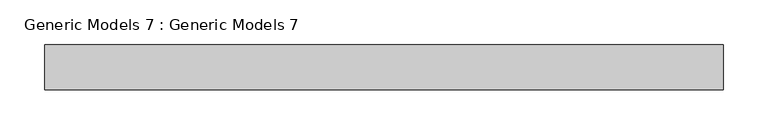
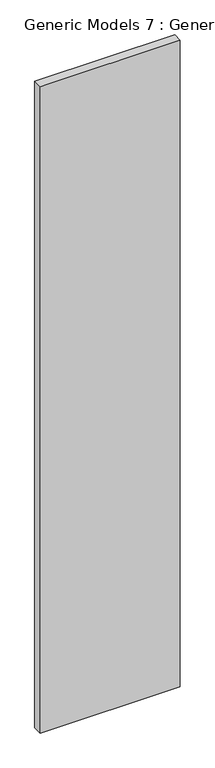
"""IFC4 building model written with IfcOpenShell, lengths in millimetres: proxy geometry, Generic Models 7 : Generic Models 7."""

from ifc_helpers import new_model, si_unit, frame, origin, place, context, project, spatial, polyline, outline, extrude, source, transform, mapped, element, save


def generic_models_7_generic_models_7_c575a30d(model_context):
    return source(origin(), model_context, "Body", "SweptSolid", [
        extrude(outline(polyline([(-5810.3607439, -6392.6842658), (-6572.3607439, -6392.6842658), (-6572.3607439, -6341.8842658), (-5810.3607439, -6341.8842658), (-5810.3607439, -6392.6842658)])), frame((0.0, 0.0, 2692.4), z_axis=(0.0, 0.0, 1.0), x_axis=(1.0, 0.0, 0.0)), (0.0, 0.0, 1.0), 3715.9761011),
    ])


if __name__ == "__main__":
    model = new_model("IFC4")
    model_context = context("Model", 3, world=origin())
    ifc_project = project(units=[si_unit("LENGTHUNIT", "METRE", prefix="MILLI")], contexts=[model_context])
    site = spatial("IfcSite", under=ifc_project)
    building = spatial("IfcBuilding", under=site)
    placement = place(None, origin())
    generic_models_7_generic_models_7_shape = generic_models_7_generic_models_7_c575a30d(model_context)
    element("IfcBuildingElementProxy", 1, Name="Generic Models 7 : Generic Models 7", ObjectType="Generic Models 7 : Generic Models 7", at=placement, inside=building, context=model_context, shape_type="MappedRepresentation", body=[
        mapped(generic_models_7_generic_models_7_shape, transform((0.0, 0.0, 0.0), x_axis=(1.0, 0.0, 0.0), y_axis=(0.0, 1.0, 0.0), z_axis=(0.0, 0.0, 1.0))),
    ])
    save(model, "model.ifc")

# Revit data of these elements
# Element 1 (IfcBuildingElementProxy, "Generic Models 7 : Generic Models 7")
#   Materials on its faces: "CLADDING WALL MATERIAL"
# Materials
#   "CLADDING WALL MATERIAL": class "Generic", colour RGB 120 120 120, transparency 0, Cost = 0
